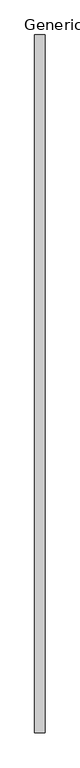
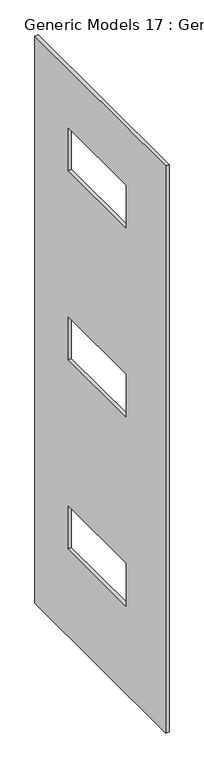
"""IFC4 building model written with IfcOpenShell, lengths in millimetres: proxy geometry, Generic Models 17 : Generic Models 17."""

from ifc_helpers import new_model, si_unit, frame, origin, place, context, project, spatial, polyline, outline, extrude, source, transform, mapped, element, save


def generic_models_17_generic_models_17_cb6d61f1(model_context):
    return source(origin(), model_context, "Body", "SweptSolid", [
        extrude(outline(polyline([(3954.6857468, 9448.8), (3954.6857468, 304.8), (499.9165128, 304.8), (499.9165128, 9448.8), (3954.6857468, 9448.8)]), holes=[polyline([(3078.0165128, 8496.2767967), (1554.0165128, 8496.2767967), (1554.0165128, 7810.4767967), (3078.0165128, 7810.4767967), (3078.0165128, 8496.2767967)]), polyline([(3078.0165128, 5448.2767967), (1554.0165128, 5448.2767967), (1554.0165128, 4762.4767967), (3078.0165128, 4762.4767967), (3078.0165128, 5448.2767967)]), polyline([(3078.0165128, 2400.2767967), (1554.0165128, 2400.2767967), (1554.0165128, 1714.4767967), (3078.0165128, 1714.4767967), (3078.0165128, 2400.2767967)])]), frame((1894.6218735, 0.0, 0.0), z_axis=(1.0, 0.0, 0.0), x_axis=(0.0, 1.0, 0.0)), (0.0, 0.0, 1.0), 50.8),
    ])


if __name__ == "__main__":
    model = new_model("IFC4")
    model_context = context("Model", 3, world=origin())
    ifc_project = project(units=[si_unit("LENGTHUNIT", "METRE", prefix="MILLI")], contexts=[model_context])
    site = spatial("IfcSite", under=ifc_project)
    building = spatial("IfcBuilding", under=site)
    placement = place(None, origin())
    generic_models_17_generic_models_17_shape = generic_models_17_generic_models_17_cb6d61f1(model_context)
    element("IfcBuildingElementProxy", 1, Name="Generic Models 17 : Generic Models 17", ObjectType="Generic Models 17 : Generic Models 17", at=placement, inside=building, context=model_context, shape_type="MappedRepresentation", body=[
        mapped(generic_models_17_generic_models_17_shape, transform((0.0, 0.0, 0.0), x_axis=(1.0, 0.0, 0.0), y_axis=(0.0, 1.0, 0.0), z_axis=(0.0, 0.0, 1.0))),
    ])
    save(model, "model.ifc")
